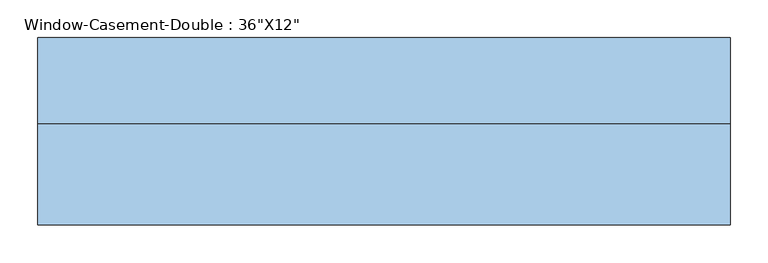
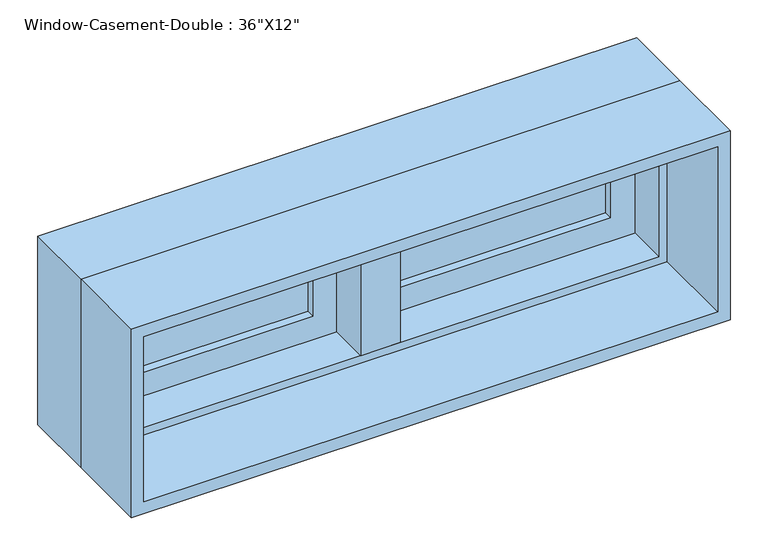
"""IFC4 building model written with IfcOpenShell, lengths in millimetres: window geometry."""

from ifc_helpers import new_model, si_unit, frame, origin, place, context, project, spatial, polyline, outline, extrude, faceted_brep, source, transform, mapped, element, save


def window_64f85577(model_context):
    return source(origin(), model_context, "Body", "SolidModel", [
        faceted_brep([(9.525, 133.35, 1206.5), (-9.525, 133.35, 1206.5), (-9.525, 82.55, 1206.5), (9.525, 82.55, 1206.5), (9.525, 133.35, 927.1), (9.525, 82.55, 927.1), (-9.525, 82.55, 927.1), (-9.525, 133.35, 927.1), (-9.525, 82.55, 946.15), (-9.525, 82.55, 1187.45), (-30.1625, 82.55, 946.15), (-30.1625, 82.55, 1187.45), (-30.1625, 19.05, 946.15), (-30.1625, 19.05, 1187.45), (30.1625, 19.05, 946.15), (30.1625, 19.05, 1187.45), (30.1625, 82.55, 946.15), (30.1625, 82.55, 1187.45), (9.525, 82.55, 946.15), (9.525, 82.55, 1187.45)], [[[0, 1, 2, 3]], [[4, 5, 6, 7]], [[1, 0, 4, 7]], [[2, 1, 7, 6, 8, 9]], [[9, 8, 10, 11]], [[11, 10, 12, 13]], [[13, 12, 14, 15]], [[15, 14, 16, 17]], [[17, 16, 18, 19]], [[0, 3, 19, 18, 5, 4]], [[18, 8, 6, 5]], [[9, 19, 3, 2]], [[8, 18, 16, 14, 12, 10]], [[19, 9, 11, 13, 15, 17]]]),
        extrude(outline(polyline([(-66.675, 114.3), (-66.675, 107.95), (-387.35, 107.95), (-387.35, 114.3), (-66.675, 114.3)])), frame((0.0, 0.0, 984.25), z_axis=(0.0, 0.0, 1.0), x_axis=(1.0, 0.0, 0.0)), (0.0, 0.0, 1.0), 165.1),
        extrude(outline(polyline([(-387.35, 95.25), (-387.35, 101.6), (-66.675, 101.6), (-66.675, 95.25), (-387.35, 95.25)])), frame((0.0, 0.0, 984.25), z_axis=(0.0, 0.0, 1.0), x_axis=(1.0, 0.0, 0.0)), (0.0, 0.0, 1.0), 165.1),
        extrude(outline(polyline([(387.35, 114.3), (387.35, 107.95), (66.675, 107.95), (66.675, 114.3), (387.35, 114.3)])), frame((0.0, 0.0, 984.25), z_axis=(0.0, 0.0, 1.0), x_axis=(1.0, 0.0, 0.0)), (0.0, 0.0, 1.0), 165.1),
        extrude(outline(polyline([(66.675, 95.25), (66.675, 101.6), (387.35, 101.6), (387.35, 95.25), (66.675, 95.25)])), frame((0.0, 0.0, 984.25), z_axis=(0.0, 0.0, 1.0), x_axis=(1.0, 0.0, 0.0)), (0.0, 0.0, 1.0), 165.1),
        extrude(outline(polyline([(1206.5, -444.5), (927.1, -444.5), (927.1, -9.525), (1206.5, -9.525), (1206.5, -444.5)]), holes=[polyline([(1149.35, -66.675), (984.25, -66.675), (984.25, -387.35), (1149.35, -387.35), (1149.35, -66.675)])]), frame((0.0, 82.55, 0.0), z_axis=(0.0, 1.0, 0.0), x_axis=(0.0, 0.0, 1.0)), (0.0, 0.0, 1.0), 44.45),
        extrude(outline(polyline([(927.1, 444.5), (1206.5, 444.5), (1206.5, 9.525), (927.1, 9.525), (927.1, 444.5)]), holes=[polyline([(984.25, 66.675), (1149.35, 66.675), (1149.35, 387.35), (984.25, 387.35), (984.25, 66.675)])]), frame((0.0, 82.55, 0.0), z_axis=(0.0, 1.0, 0.0), x_axis=(0.0, 0.0, 1.0)), (0.0, 0.0, 1.0), 44.45),
        extrude(outline(polyline([(1219.2, -457.2), (914.4, -457.2), (914.4, 457.2), (1219.2, 457.2), (1219.2, -457.2)]), holes=[polyline([(1200.15, 438.15), (933.45, 438.15), (933.45, -438.15), (1200.15, -438.15), (1200.15, 438.15)])]), frame((0.0, -114.3, 0.0), z_axis=(0.0, 1.0, 0.0), x_axis=(0.0, 0.0, 1.0)), (0.0, 0.0, 1.0), 133.35),
        faceted_brep([(425.45, 82.55, 1187.45), (425.45, 19.05, 1187.45), (-425.45, 19.05, 1187.45), (-425.45, 82.55, 1187.45), (444.5, 133.35, 1206.5), (444.5, 82.55, 1206.5), (-444.5, 82.55, 1206.5), (-444.5, 133.35, 1206.5), (457.2, 19.05, 1219.2), (457.2, 133.35, 1219.2), (-457.2, 133.35, 1219.2), (-457.2, 19.05, 1219.2), (-425.45, 19.05, 946.15), (-425.45, 82.55, 946.15), (-444.5, 82.55, 927.1), (-444.5, 133.35, 927.1), (-457.2, 133.35, 914.4), (-457.2, 19.05, 914.4), (425.45, 19.05, 946.15), (425.45, 82.55, 946.15), (444.5, 82.55, 927.1), (444.5, 133.35, 927.1), (457.2, 133.35, 914.4), (457.2, 19.05, 914.4)], [[[0, 1, 2, 3]], [[4, 5, 6, 7]], [[8, 9, 10, 11]], [[3, 2, 12, 13]], [[7, 6, 14, 15]], [[11, 10, 16, 17]], [[13, 12, 18, 19]], [[15, 14, 20, 21]], [[17, 16, 22, 23]], [[11, 17, 23, 8], [1, 18, 12, 2]], [[19, 18, 1, 0]], [[5, 20, 14, 6], [3, 13, 19, 0]], [[21, 20, 5, 4]], [[23, 22, 9, 8]], [[9, 22, 16, 10], [7, 15, 21, 4]]]),
    ])


if __name__ == "__main__":
    model = new_model("IFC4")
    model_context = context("Model", 3, world=origin())
    ifc_project = project(units=[si_unit("LENGTHUNIT", "METRE", prefix="MILLI")], contexts=[model_context])
    site = spatial("IfcSite", under=ifc_project)
    building = spatial("IfcBuilding", under=site)
    placement = place(None, origin())
    window_shape = window_64f85577(model_context)
    element("IfcWindow", 1, ObjectType="Window-Casement-Double : 36\"X12\"", at=placement, inside=building, context=model_context, shape_type="MappedRepresentation", body=[
        mapped(window_shape, transform((0.0, 0.0, 0.0), x_axis=(1.0, 0.0, 0.0), y_axis=(0.0, 1.0, 0.0), z_axis=(0.0, 0.0, 1.0))),
    ])
    save(model, "model.ifc")

# Revit data of these elements
# Type "Window-Casement-Double : 36\"X12\""
#   Type Mark = "24"
#   Fire Rating = "0.5h"
#   Assembly Code = "B2020100"
#   Analytic Construction = "Double glazing - domestic"
#   Frame Extension [instance default] = 0' - 0 1/4"
#   Window Inset [instance default] = 0' - 0"
#   Wall Thickness [instance default] = 0' - 6"
#   Interior Wall Closure [instance default] = 0' - 2 1/4"
#   Half Width = 1' - 6"
#   Visual Light Transmittance = 0.81
#   Thermal Resistance (R) = 1.8146 (h·ft²·°F)/BTU
#   Solar Heat Gain Coefficient = 0.76
#   Rough Width = 3' - 0 1/2"
#   Rough Height = 1' - 0 1/2"
#   Height = 1' - 0"
#   Heat Transfer Coefficient (U) = 0.5511 BTU/(h·ft²·°F)
#   Exterior Wall Closure [instance default] = 0' - 1 1/4"
#   Extension Jamb [instance default] = 0' - 2 1/4"
#   Default Sill Height = 3' - 0"
#   Width = 3' - 0"
#   Muntin Visibility = yes
#   Interior Trim Visibility [instance default] = yes
#   Exterior Trim Visibility [instance default] = yes
#   Extension Jamb Visibility [instance default] = yes
#   Interior Trim Material = Wood - Stained
#   Muntin Pattern = Muntin Pattern_2x2 : Muntin Pattern_2x2
#   Interior Trim = Trim-Window-Interior-Flat : Picture Frame
#   Interior Frame Material = Wood - Stained
#   Glass Panel Material = Glass
#   Exterior Trim Material = Clad - White
#   Exterior Trim = Trim-Window-Exterior-Flat : with Sill
#   Exterior Frame Material = Clad - White
#   Wall Closure = (empty or 0)
# Element 1 (IfcWindow, "Window-Casement-Double : 36\"X12\"")
#   Wall Thickness = 0' - 9"
#   Extension Jamb = 0' - 5 1/4"
#   Materials on its faces: "Wood - Stained", "Glass", "Clad - White"
# Materials
#   "Wood - Stained": class "Wood", colour RGB 224 178 126, transparency 0, Cost = 0
#   "Glass": class "Glass", colour RGB 0 128 192, transparency 0.75, Description = "Soda Lime Glass", Cost = 0
#   "Clad - White": class "Wood", colour RGB 242 242 238, transparency 0, Cost = 0
